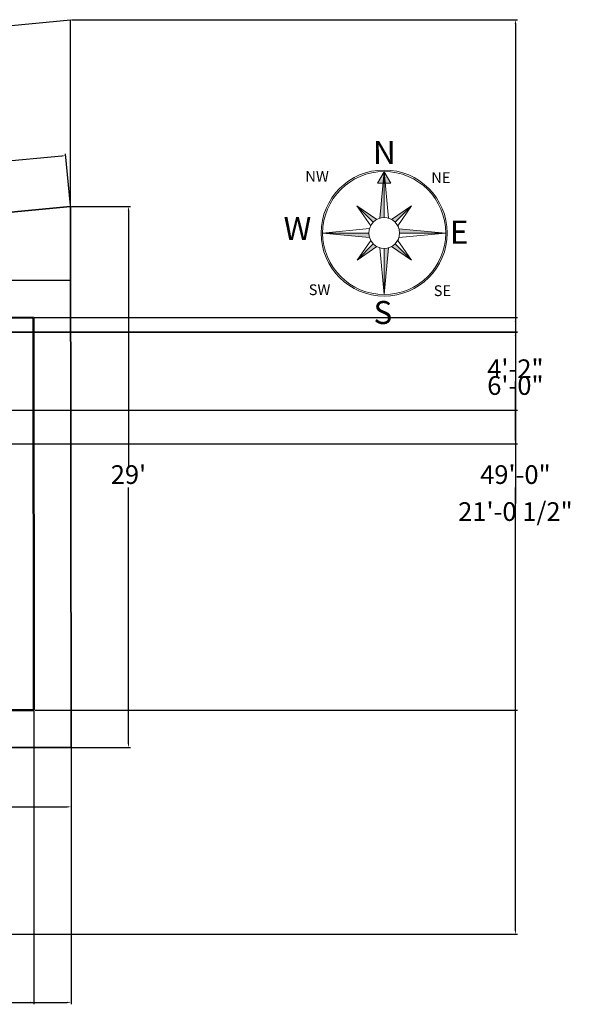
# Model space of a CAD drawing. Units: inches. Extents: x 5307 to 6359, y 4763 to 5474.
# Tile 5 of 5: x 6006 to 6359, y 4773 to 5406. Entities that reach past the tile are written whole.
import ezdxf

# ---------------------------------------------------------------- set-up
doc = ezdxf.new("R2010")
doc.units = ezdxf.units.IN
for name, color, linetype, lineweight in [('A-ANNO-DIMS', 2, 'Continuous', 18), ('A-ANNO-SYMB', 7, 'Continuous', 18), ('A-WALL', 7, 'Continuous', 50), ('C-PROP', 7, 'Continuous', 35), ('ROAD', 240, 'Continuous', 25)]:
    doc.layers.add(name, color=color, linetype=linetype, lineweight=lineweight)
doc.styles.add('A', font='txt', dxfattribs={"height": 200})
doc.styles.get("Standard").update_dxf_attribs({"font": 'arial.ttf'})
doc.dimstyles.new('ISO-25', dxfattribs={"dimtxt": 12, "dimasz": 2.5, "dimexe": 1.25, "dimexo": 0.625, "dimtad": 1, "dimtih": 1, "dimtoh": 1, "dimlunit": 4, "dimtxsty": 'Standard', "dimcen": 2.5, "dimadec": 0, "dimazin": 0, "dimtfac": 1, "dimtmove": 0, "dimatfit": 3, "dimfxl": 1, "dimarcsym": 0})

# ---------------------------------------------------------------- blocks, each defined once
blk = doc.blocks.new('*D1')
at = {"layer": 'A-ANNO-DIMS', "color": 0, "lineweight": -2, "transparency": 16777216}
for p, q in [((6038.88, 5285.78), (6076.67, 5285.78)), ((6075.42, 5283.28), (6075.42, 5118.54)), ((6075.42, 4940.28), (6075.42, 5105.03)), ((6038.88, 4937.78), (6076.67, 4937.78))]:
    blk.add_line(p, q, dxfattribs=at)
at = {"layer": 'A-ANNO-DIMS', "color": 0, "transparency": 16777216}
for points in [[(6075, 5283.28), (6075.84, 5283.28), (6075.42, 5285.78)], [(6075, 4940.28), (6075.84, 4940.28), (6075.42, 4937.78)]]:
    blk.add_solid(points, dxfattribs=at)
at = {"layer": 'Defpoints', "color": 0, "transparency": 16777216}
for p in [(6038.25, 5285.78), (6075.42, 5285.78), (6038.25, 4937.78)]:
    blk.add_point(p, dxfattribs=at)
at = {"layer": 'A-ANNO-DIMS', "color": 0, "transparency": 16777216, "insert": (6075.42, 5111.78), "char_height": 12, "attachment_point": 5}
blk.add_mtext("29'", dxfattribs=at)
blk = doc.blocks.new('*D2')
at = {"layer": 'A-ANNO-DIMS', "color": 0, "lineweight": -2, "transparency": 16777216}
for p, q in [((6032.58, 5318.14), (5810.72, 5296.48)), ((6038.19, 5286.41), (6034.95, 5319.62)), ((5545.9, 5270.62), (5767.76, 5292.28)), ((5546.53, 5238.41), (5543.29, 5271.62))]:
    blk.add_line(p, q, dxfattribs=at)
at = {"layer": 'A-ANNO-DIMS', "color": 0, "transparency": 16777216}
for points in [[(6032.54, 5318.55), (6032.62, 5317.72), (6035.07, 5318.38)], [(5545.86, 5271.04), (5545.94, 5270.21), (5543.41, 5270.38)]]:
    blk.add_solid(points, dxfattribs=at)
at = {"layer": 'Defpoints', "color": 0, "transparency": 16777216}
for p in [(6035.07, 5318.38), (6038.25, 5285.78), (5546.59, 5237.78)]:
    blk.add_point(p, dxfattribs=at)
at = {"layer": 'A-ANNO-DIMS', "color": 0, "transparency": 16777216, "insert": (5789.24, 5294.38), "char_height": 12, "attachment_point": 5}
blk.add_mtext('41\'-2"', dxfattribs=at)
blk = doc.blocks.new('*D4')
at = {"layer": 'A-ANNO-DIMS', "color": 0, "lineweight": -2, "transparency": 16777216}
for p, q in [((6038.59, 4937.64), (6038.59, 4898.47)), ((5546.59, 4937.16), (5546.59, 4898.47)), ((5549.09, 4899.72), (6036.09, 4899.72))]:
    blk.add_line(p, q, dxfattribs=at)
at = {"layer": 'A-ANNO-DIMS', "color": 0, "transparency": 16777216}
for points in [[(5549.09, 4900.14), (5549.09, 4899.3), (5546.59, 4899.72)], [(6036.09, 4900.14), (6036.09, 4899.3), (6038.59, 4899.72)]]:
    blk.add_solid(points, dxfattribs=at)
at = {"layer": 'Defpoints', "color": 0, "transparency": 16777216}
for p in [(5546.59, 4937.78), (6038.59, 4938.26), (6038.59, 4899.72)]:
    blk.add_point(p, dxfattribs=at)
at = {"layer": 'A-ANNO-DIMS', "color": 0, "transparency": 16777216, "insert": (5792.59, 4906.37), "char_height": 12, "attachment_point": 5}
blk.add_mtext("41'", dxfattribs=at)
blk = doc.blocks.new('A$C4C25277F')
for points in [[(22.44, 27.36, -0.072542), (23.47, 27.49), (23.7, 38.36)], [(17.12, 30.4), (20.25, 25.65, -0.072542), (20.89, 26.48)], [(29.94, 30.14), (26.62, 25.52, 0.072542), (26.02, 26.37)], [(8.94, 24.16), (8.94, 24.16), (11.65, 23.84), (11.66, 24.1)], [(11.66, 24.1), (11.65, 23.84), (19.9, 22.9, -0.072542), (19.78, 23.94)], [(26.9, 24.82, -0.072542), (27.02, 23.79), (37.9, 23.56)], [(16.86, 17.58), (20.18, 22.2, 0.072542), (20.78, 21.35)], [(29.68, 17.32), (26.55, 22.07, -0.072542), (25.91, 21.24)], [(24.36, 20.37, -0.072542), (23.33, 20.24), (23.1, 9.36)]]:
    blk.add_hatch(color=256).paths.add_polyline_path(points)
h = blk.add_hatch(color=256)
h.dxf.hatch_style = 1
h.paths.add_polyline_path([(8.95, 24.16), (11.66, 24.36), (11.69, 25.67)])
h.paths.add_polyline_path([(8.94, 24.16), (11.62, 22.53), (11.65, 23.84)])
h.paths.add_polyline_path([(11.66, 24.1), (11.66, 24.36), (8.95, 24.16), (8.94, 24.16)])
for p, q in [((23.7, 38.36), (22.44, 27.36)), ((23.7, 38.36), (23.47, 27.49)), ((23.7, 38.36), (24.51, 27.31)), ((17.12, 30.4), (21.74, 27.08)), ((17.12, 30.4), (20.25, 25.65)), ((17.12, 30.4), (20.89, 26.48)), ((29.94, 30.14), (25.19, 27.01)), ((29.94, 30.14), (26.02, 26.37)), ((29.94, 30.14), (26.62, 25.52)), ((11.69, 25.67), (8.94, 24.16)), ((11.62, 22.53), (11.69, 25.67)), ((8.9, 24.16), (19.95, 24.97)), ((8.9, 24.16), (19.78, 23.94)), ((8.9, 24.16), (19.9, 22.9)), ((8.9, 24.16), (9.81, 24.14)), ((8.94, 24.16), (11.62, 22.53)), ((37.9, 23.56), (26.85, 22.75)), ((37.9, 23.56), (26.9, 24.82)), ((37.9, 23.56), (27.02, 23.79)), ((16.86, 17.58), (20.18, 22.2)), ((16.86, 17.58), (20.78, 21.35)), ((29.68, 17.32), (25.91, 21.24)), ((29.68, 17.32), (26.55, 22.07)), ((16.86, 17.58), (21.61, 20.71)), ((23.1, 9.36), (22.29, 20.41)), ((23.1, 9.36), (24.36, 20.37)), ((23.1, 9.36), (23.33, 20.24)), ((29.68, 17.32), (25.06, 20.64))]:
    blk.add_line(p, q)
for radius in [14.86, 14.5, 3.63]:
    blk.add_circle((23.4, 23.86), radius)
at = {"style": 'A'}
for s, height, p in [('E', 5.44, (26.25, 39.3)), ('NE', 2.538, (11.84, 35.19)), ('SE', 2.538, (38.5, 35.21)), ('N', 5.44, (7.06, 21.55)), ('S', 5.44, (44.8, 20.9)), ('NW', 2.538, (10.94, 5.53)), ('SW', 2.538, (37.67, 5.77)), ('W', 5.44, (24.58, 0.13))]:
    blk.add_text(s, height=height, rotation=88.8164, dxfattribs=at).set_placement(p)
blk = doc.blocks.new('*D12')
at = {"layer": 'A-ANNO-DIMS', "color": 0, "lineweight": -2, "transparency": 16777216}
for p, q in [((6038.59, 4937.16), (6038.59, 4772.78)), ((5426.59, 4817.16), (5426.59, 4772.78)), ((5429.09, 4774.03), (6036.09, 4774.03))]:
    blk.add_line(p, q, dxfattribs=at)
at = {"layer": 'A-ANNO-DIMS', "color": 0, "transparency": 16777216}
for points in [[(5429.09, 4774.45), (5429.09, 4773.62), (5426.59, 4774.03)], [(6036.09, 4774.45), (6036.09, 4773.62), (6038.59, 4774.03)]]:
    blk.add_solid(points, dxfattribs=at)
at = {"layer": 'Defpoints', "color": 0, "transparency": 16777216}
for p in [(6038.59, 4937.78), (5426.59, 4817.78), (6038.59, 4774.03)]:
    blk.add_point(p, dxfattribs=at)
at = {"layer": 'A-ANNO-DIMS', "color": 0, "transparency": 16777216, "insert": (5732.59, 4780.79), "char_height": 12, "attachment_point": 5}
blk.add_mtext('51\'-0"', dxfattribs=at)
blk = doc.blocks.new('*D13')
at = {"layer": 'A-ANNO-DIMS', "color": 0, "lineweight": -2, "transparency": 16777216}
for p, q in [((6038.88, 5405.78), (6325.25, 5405.78)), ((6324, 5403.28), (6324, 5118.54)), ((6324, 4820.28), (6324, 5105.03)), ((5547.22, 4817.78), (6325.25, 4817.78))]:
    blk.add_line(p, q, dxfattribs=at)
at = {"layer": 'A-ANNO-DIMS', "color": 0, "transparency": 16777216}
for points in [[(6323.58, 5403.28), (6324.41, 5403.28), (6324, 5405.78)], [(6323.58, 4820.28), (6324.41, 4820.28), (6324, 4817.78)]]:
    blk.add_solid(points, dxfattribs=at)
at = {"layer": 'Defpoints', "color": 0, "transparency": 16777216}
for p in [(6038.25, 5405.78), (6324, 5405.78), (5546.59, 4817.78)]:
    blk.add_point(p, dxfattribs=at)
at = {"layer": 'A-ANNO-DIMS', "color": 0, "transparency": 16777216, "insert": (6324, 5111.78), "char_height": 12, "attachment_point": 5}
blk.add_mtext('49\'-0"', dxfattribs=at)
blk = doc.blocks.new('*D31')
at = {"layer": 'A-ANNO-DIMS', "color": 0, "lineweight": -2, "transparency": 16777216}
for p, q in [((5704.72, 5204.94), (6325.25, 5204.94)), ((6324, 5202.44), (6324, 5186.48)), ((6324, 5157.23), (6324, 5173.19)), ((5704.72, 5154.73), (6325.25, 5154.73))]:
    blk.add_line(p, q, dxfattribs=at)
at = {"layer": 'A-ANNO-DIMS', "color": 0, "transparency": 16777216}
for points in [[(6323.58, 5202.44), (6324.41, 5202.44), (6324, 5204.94)], [(6323.58, 5157.23), (6324.41, 5157.23), (6324, 5154.73)]]:
    blk.add_solid(points, dxfattribs=at)
at = {"layer": 'Defpoints', "color": 0, "transparency": 16777216}
for p in [(5704.09, 5204.94), (6324, 5204.94), (5704.09, 5154.73)]:
    blk.add_point(p, dxfattribs=at)
at = {"layer": 'A-ANNO-DIMS', "color": 0, "transparency": 16777216, "insert": (6324, 5179.83), "char_height": 12, "attachment_point": 5}
blk.add_mtext('4\'-2"', dxfattribs=at)
blk = doc.blocks.new('*D32')
at = {"layer": 'A-ANNO-DIMS', "color": 0, "lineweight": -2, "transparency": 16777216}
for p, q in [((5809.46, 5205.04), (6325.25, 5205.04)), ((6324, 5202.54), (6324, 5175.79)), ((6324, 5135.54), (6324, 5162.29)), ((5809.53, 5133.04), (6325.25, 5133.04))]:
    blk.add_line(p, q, dxfattribs=at)
at = {"layer": 'A-ANNO-DIMS', "color": 0, "transparency": 16777216}
for points in [[(6323.58, 5202.54), (6324.41, 5202.54), (6324, 5205.04)], [(6323.58, 5135.54), (6324.41, 5135.54), (6324, 5133.04)]]:
    blk.add_solid(points, dxfattribs=at)
at = {"layer": 'Defpoints', "color": 0, "transparency": 16777216}
for p in [(5808.83, 5205.04), (6324, 5205.04), (5808.9, 5133.04)]:
    blk.add_point(p, dxfattribs=at)
at = {"layer": 'A-ANNO-DIMS', "color": 0, "transparency": 16777216, "insert": (6324, 5169.04), "char_height": 12, "attachment_point": 5}
blk.add_mtext('6\'-0"', dxfattribs=at)
blk = doc.blocks.new('*D33')
at = {"layer": 'A-ANNO-DIMS', "color": 0, "lineweight": -2, "transparency": 16777216}
for p, q in [((5570.59, 4961.16), (5570.59, 4772.78)), ((6014.57, 4961.16), (6014.57, 4772.78)), ((5573.09, 4774.03), (6012.07, 4774.03))]:
    blk.add_line(p, q, dxfattribs=at)
at = {"layer": 'A-ANNO-DIMS', "color": 0, "transparency": 16777216}
for points in [[(5573.09, 4774.45), (5573.09, 4773.62), (5570.59, 4774.03)], [(6012.07, 4774.45), (6012.07, 4773.62), (6014.57, 4774.03)]]:
    blk.add_solid(points, dxfattribs=at)
at = {"layer": 'Defpoints', "color": 0, "transparency": 16777216}
for p in [(5570.59, 4961.78), (6014.57, 4961.78), (6014.57, 4774.03)]:
    blk.add_point(p, dxfattribs=at)
at = {"layer": 'A-ANNO-DIMS', "color": 0, "transparency": 16777216, "insert": (5792.58, 4780.79), "char_height": 12, "attachment_point": 5}
blk.add_mtext('37\'-0"', dxfattribs=at)
blk = doc.blocks.new('*D34')
at = {"layer": 'A-ANNO-DIMS', "color": 0, "lineweight": -2, "transparency": 16777216}
for p, q in [((6014.95, 5214.24), (6325.25, 5214.24)), ((6324, 5211.74), (6324, 5094.84)), ((6324, 4964.28), (6324, 5081.18)), ((6015.19, 4961.78), (6325.25, 4961.78))]:
    blk.add_line(p, q, dxfattribs=at)
at = {"layer": 'A-ANNO-DIMS', "color": 0, "transparency": 16777216}
for points in [[(6323.58, 5211.74), (6324.41, 5211.74), (6324, 5214.24)], [(6323.58, 4964.28), (6324.41, 4964.28), (6324, 4961.78)]]:
    blk.add_solid(points, dxfattribs=at)
at = {"layer": 'Defpoints', "color": 0, "transparency": 16777216}
for p in [(6014.32, 5214.24), (6324, 5214.24), (6014.57, 4961.78)]:
    blk.add_point(p, dxfattribs=at)
at = {"layer": 'A-ANNO-DIMS', "color": 0, "transparency": 16777216, "insert": (6324, 5088.01), "char_height": 12, "attachment_point": 5}
blk.add_mtext('21\'-0 1/2"', dxfattribs=at)

msp = doc.modelspace()

# ---------------------------------------------------------------- linework, layer by layer
at = {"layer": 'A-WALL'}
for p, q in [((5570.592, 5213.807), (6014.324, 5214.238)), ((6014.569, 4961.784), (6014.324, 5214.238)), ((6014.56, 4970.784), (6014.569, 4970.784)), ((5570.592, 4961.784), (6014.569, 4961.784)), ((6005.569, 4961.775), (6005.569, 4961.784))]:
    msp.add_line(p, q, dxfattribs=at)
at = {"layer": 'C-PROP'}
for p, q in [((6038.255, 5285.784), (5546.592, 5237.784)), ((6038.592, 4937.784), (6038.255, 5285.784)), ((5546.592, 5237.784), (6038.301, 5238.261)), ((6038.569, 4961.784), (6038.592, 4961.784)), ((5546.592, 4937.784), (6038.592, 4937.784)), ((6014.592, 4937.761), (6014.592, 4937.784))]:
    msp.add_line(p, q, dxfattribs=at)
at = {"layer": 'ROAD'}
for p in [(5546.592, 5357.784), (6038.255, 5285.784)]:
    msp.add_line(p, (6038.255, 5405.784), dxfattribs=at)

# ---------------------------------------------------------------- block references
at = {"layer": 'A-ANNO-SYMB', "xscale": 2.726477399694939, "yscale": 2.726477399694939, "zscale": 2.726477399694939, "rotation": 271.1835448777349}
msp.add_blockref('A$C4C25277F', (6173.359, 5331.062), dxfattribs=at)

# ---------------------------------------------------------------- dimensions: what is measured, and where the dimension line sits
at = {"layer": 'A-ANNO-DIMS'}
for base, p1, p2, override, picture, middle in [((6323.996, 5405.784), (5546.592, 4817.784), (6038.255, 5405.784), {"dimdec": 1, "dimlfac": 1, "dimrnd": 0, "dimzin": 1, "dimdsep": 46, "dimlunit": 4, "dimfrac": 2}, '*D13', (6323.996, 5111.784)), ((6075.42, 5285.784), (6038.255, 4937.784), (6038.255, 5285.784), {"dimclrd": 0, "dimclre": 0, "dimclrt": 0}, '*D1', (6075.42, 5111.784)), ((6323.996, 5214.238), (6014.569, 4961.784), (6014.324, 5214.238), {"dimdec": 1, "dimlfac": 1, "dimrnd": 0, "dimzin": 1, "dimdsep": 46, "dimlunit": 4, "dimfrac": 2}, '*D34', (6323.996, 5088.011)), ((6323.996, 5204.937), (5704.092, 5154.733), (5704.092, 5204.937), {"dimdec": 1, "dimlfac": 1, "dimrnd": 0, "dimzin": 1, "dimdsep": 46, "dimlunit": 4, "dimfrac": 2}, '*D31', (6323.996, 5179.835)), ((6323.996, 5205.038), (5808.903, 5133.038), (5808.833, 5205.038), {"dimdec": 1, "dimlfac": 1, "dimrnd": 0, "dimzin": 1, "dimdsep": 46, "dimlunit": 4, "dimfrac": 2}, '*D32', (6323.996, 5169.038))]:
    dim = msp.add_linear_dim(base=base, p1=p1, p2=p2, angle=90, dimstyle='ISO-25', override=override, dxfattribs=at)
    dim.commit()
    dim.dimension.update_dxf_attribs({"geometry": picture, "text_midpoint": middle})
dim = msp.add_aligned_dim(p1=(5546.592, 5237.784), p2=(6038.255, 5285.784), distance=32.752, dimstyle='ISO-25', override={"dimclrd": 0, "dimclre": 0, "dimclrt": 0}, dxfattribs=at)
dim.commit()
dim.dimension.update_dxf_attribs({"geometry": '*D2', "text_midpoint": (5789.241, 5294.381)})
for base, p1, p2, override, picture, middle in [((6014.569, 4774.034), (5570.592, 4961.784), (6014.569, 4961.784), {"dimdec": 1, "dimlfac": 1, "dimrnd": 0, "dimzin": 1, "dimdsep": 46, "dimlunit": 4, "dimfrac": 2}, '*D33', (5792.581, 4780.79)), ((6038.592, 4774.034), (5426.592, 4817.784), (6038.592, 4937.784), {"dimdec": 1, "dimlfac": 1, "dimrnd": 0, "dimzin": 1, "dimdsep": 46, "dimlunit": 4, "dimfrac": 2}, '*D12', (5732.592, 4780.786)), ((6038.592, 4899.719), (5546.592, 4937.784), (6038.592, 4938.261), {"dimclrd": 0, "dimclre": 0, "dimclrt": 0}, '*D4', (5792.592, 4906.368))]:
    dim = msp.add_linear_dim(base=base, p1=p1, p2=p2, dimstyle='ISO-25', override=override, dxfattribs=at)
    dim.commit()
    dim.dimension.update_dxf_attribs({"geometry": picture, "text_midpoint": middle})

doc.saveas('drawing.dxf')
